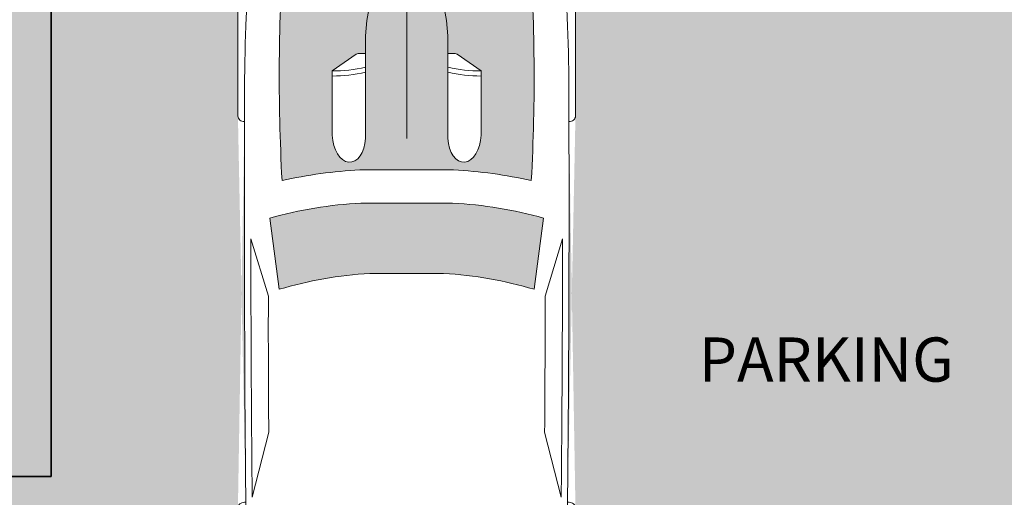
# Model space of a CAD drawing. Units: inches. Extents: x 2549 to 3108, y 1683 to 2362.
# Tile 5 of 30: x 2877 to 3018, y 1793 to 1861. Entities that reach past the tile are written whole.
import ezdxf

# ---------------------------------------------------------------- set-up
doc = ezdxf.new("R2010")
doc.units = ezdxf.units.IN
for name, color, linetype, lineweight in [('A-ANNO-DIMS', 2, 'Continuous', 18), ('A-AREA-IDEN', 7, 'Continuous', 18), ('A-FURN-PATT', 9, 'Continuous', 13), ('A-WALL', 7, 'Continuous', 35), ('A-WALL-PATT', 89, 'Continuous', 13), ('C-PKNG-VEHI', 8, 'Continuous', 18)]:
    doc.layers.add(name, color=color, linetype=linetype, lineweight=lineweight)
doc.layers.add('C-PKNG-VEHI-PATT', color=251, linetype='Continuous', lineweight=13, true_color=0x636466)
doc.layers.add('C-PVMT-PATT', color=9, linetype='Continuous', lineweight=13, true_color=0xc7c8ca)
doc.styles.get("Standard").update_dxf_attribs({"font": 'arial.ttf'})
doc.dimstyles.get("Standard").update_dxf_attribs({"dimtxt": 0.18, "dimasz": 0.18, "dimexe": 0.18, "dimexo": 0.0625, "dimgap": 0.09, "dimtad": 0, "dimtih": 1, "dimtoh": 1, "dimdec": 4, "dimzin": 0, "dimdsep": 46, "dimtxsty": 'Standard', "dimcen": 0.09, "dimadec": 0, "dimazin": 0, "dimtfac": 1, "dimtdec": 4, "dimtofl": 0, "dimtmove": 0, "dimatfit": 3, "dimfxl": 1, "dimtolj": 1, "dimtzin": 0, "dimarcsym": 0})

# ---------------------------------------------------------------- blocks, each defined once
blk = doc.blocks.new('*U11')
for p, q in [((46.55368679439944, 38.88847654282876), (22.35054758993934, 38.88847654282876)), ((136.6978032355602, 38.88847654282876), (160.90094244002, 38.88847654282867)), ((21.10406751471477, 37.40863046792069), (21.10406751471477, 36.83230215753705)), ((47.80016686962392, 37.39011648242055), (47.80016686962392, 37.40863046792069)), ((135.4513231603356, 37.07354110333037), (135.4513231603356, 37.40863046792069)), ((162.1474225152445, 37.40863046792049), (162.1474225152445, 36.77402019194128)), ((87.98532186932616, 31.87120872459877), (74.75900729854769, 35.92175679182955)), ((134.313356548143, 35.6043097713567), (119.2882629232503, 31.77757799177584)), ((186.4728846989705, -33.49860931502491), (186.4728846989718, 33.49860931502465)), ((188.3990091454065, -32.75868627757393), (188.3990091454077, 32.75868627757058)), ((70.0302824853563, 31.53613089391356), (86.40615155322342, 29.35124891408057)), ((138.4228833961707, 29.35124891408074), (157.2465674415997, 29.35124891408074)), ((186.4728846989718, 29.35124891408083), (167.0083537481071, 29.35124891408083)), ((164.515393597658, 26.39155676426461), (164.5153935976578, -26.39155676426503)), ((32.26591480791686, 11.62530558863241), (36.12873726252356, 17.16961494239206)), ((36.12873726252356, 17.16961494239206), (50.93891189819171, 17.16961494239206)), ((29.77279020470884, 9.505833383620029), (51.68362801571248, 9.505833383620029)), ((32.12291633764599, 9.505833383620029), (32.12291633764599, 11.15369945057711)), ((58.9167604809788, -10.77488335095668), (58.9167604809788, 10.77488335095617)), ((66.55009204259746, -10.5288681329018), (66.55009204259746, 10.52886813290129)), ((186.4728846989718, -10.5288681329018), (186.4728846989718, 10.52886813290129)), ((82.73706193978568, 8.496039918672748), (82.73706193978568, -8.49603991867258)), ((3.266462181856987, 6.128290093440767), (0.1022408397004821, 0.4060708604429806)), ((-4.43e-14, -2.558e-13), (51.68362801571248, -2.558e-13)), ((0.1022408397004821, -0.4060708604432933), (3.266462181856987, -6.128290093441194)), ((29.77279020470884, -9.50583338362054), (51.68362801571248, -9.50583338362054)), ((32.12291633764599, -9.50583338362054), (32.12291633764599, -11.15369945057762)), ((32.26591480791686, -11.62530558863292), (36.12873726252356, -17.16961494239257)), ((36.12873726252356, -17.16961494239257), (50.93891189819171, -17.16961494239257)), ((86.40615155322318, -29.35124891408145), (70.03028248535594, -31.53613089391442)), ((157.2465674415997, -29.35124891408117), (138.4228833961707, -29.35124891408126)), ((167.008353748107, -29.35124891408126), (186.4728846989707, -29.35124891408108)), ((87.98532186932607, -31.87120872459903), (74.7590072985476, -35.92175679182964)), ((134.3133565481428, -35.60430977135721), (119.2882629232503, -31.77757799177618)), ((21.10406751471477, -37.4086304679212), (21.10406751471477, -36.83230215753756)), ((47.80016686962392, -37.39011648242107), (47.80016686962392, -37.4086304679212)), ((135.4513231603355, -37.07354110333088), (135.4513231603355, -37.4086304679212)), ((162.1474225152445, -37.408630467921), (162.1474225152445, -36.77402019194179)), ((46.55368679439944, -38.88847654282927), (22.35054758993934, -38.88847654282927)), ((136.6978032355602, -38.88847654282927), (160.9009424400199, -38.88847654282918))]:
    blk.add_line(p, q)
for centre, major_axis, ratio, start_param, end_param in [((22.35054758993934, 37.40863046792072), (2.08e-14, -1.479846074908118), 0.842303869543976, 3.141592653589776, 4.712388980384677), ((46.55368679439944, 37.40863046792072), (2.2e-14, 1.479846074908118), 0.8423038695439758, -1.570796326794884, 1.73e-14), ((136.6978032355602, 37.40863046792072), (2.357e-13, -1.479846074908118), 0.842303869543976, 3.141592653589603, 4.712388980384554), ((160.90094244002, 37.40863046792052), (5.59e-14, 1.479846074908118), 0.842303869543976, -1.570796326794865, 4.44e-14), ((41.19115208863305, -490.8631038926156), (1.294e-13, 528.2339998381949), 0.8423038695439741, 0.0028100083536837, 0.0755983031096952), ((64.48199294511879, -10555.61767587835), (1.907644e-10, 10593.02630634627), 0.842303869543847, -0.0133969486112073, 0.0027970409639888), ((180.6280394947615, 35.8381667808375), (7.4e-14, 2.219769112362114), 0.8423038695439693, -0.0130174256259048, 1.249894140392862), ((64.48199294754608, -10556.35759891604), (1.349839377e-06, 10595.3130398087), 0.8423038681351469, -0.0133969484821159, -0.0130174254969711), ((183.9799245485226, 33.49860931502124), (3e-16, -2.959692149816168), 0.8423038695439952, 1.570796326796048, 3.128195704978389), ((183.9799245485216, 32.75868627756583), (8.56e-14, -5.246425615115243), 0.8423038695439737, 1.570796326795794, 3.128195704978164), ((266.0300214172791, -27.52442688366631), (1.966072e-10, 313.3077612809058), 0.8423038695435284, 1.367075990158062, 1.391760499156098), ((64.4819929449925, -10555.61767590795), (1.9177683e-09, -10591.54646030096), 0.8423038695482963, 3.133765086725325, 3.140440689641252), ((95.78879860270445, -3666.353346297651), (1.949864e-10, -3698.236159209632), 0.8423038695446962, 3.134048706297306, 3.14409775411291), ((37.47375371777758, -593.9621830607928), (6.21e-14, -623.32820996736), 0.8423038695439826, 3.09604606856106, 3.200911180495224), ((135.2911776514449, 5.387441675478555), (2.2715e-12, 81.77258453065997), 0.8423038695439563, 1.245306111696802, 1.507880129813836), ((259.1750197310735, -27.52442688366614), (1.506617e-10, -305.3028914627677), 0.8423038695443789, 4.528606069860317, 4.561837674556238), ((134.4003789125686, 5.387441675477674), (4.276e-13, -89.7774543484738), 0.84230386954398, 4.44948196380473, 4.652344057257214), ((149.595361812917, 2.799442537139299), (8.561e-13, -79.57966406425402), 0.842303869543983, 4.372215489277867, 4.640744122441986), ((17.08207736189386, -1.421e-13), (6.87e-14, 147.0179238898305), 0.8423038695439764, 4.511394369635731, 4.913383591133647), ((35.90576140732288, -1.421e-13), (6.87e-14, 147.0179238898305), 0.8423038695439764, 4.511394369635731, 4.913383591133647), ((167.0083537481071, 26.39155676426464), (1.394e-13, 2.959692149816236), 0.842303869543976, 5.55e-14, 1.57079632679492), ((-204.4946649195746, 52.39684969293512), (4.12053e-11, -250.9602162198571), 0.8423038695441164, 1.385369446298923, 1.434372047871027), ((13.03653510440275, 17.00972444508943), (1.2303e-12, 27.41599049210566), 0.8423038695439277, 4.435146050259648, 4.718221029521873), ((14.20086229321332, 17.00972444508943), (1.2303e-12, 27.41599049210566), 0.8423038695439277, 4.435146050259648, 4.718221029521873), ((50.7902773840875, 13.33772416300607), (6.340077547122382, -0.356608581037027), 0.6038335755719145, -1.39555193967809, 1.581314658479915), ((32.74615637525823, 11.15369945057713), (1.313e-13, 0.7399230374541176), 0.8423038695439091, 0.8797135699495516, 1.570796326795045), ((29.77279020470884, -46.66302566589627), (5.12e-14, 56.16885904951626), 0.842303869543976, 7e-16, 0.5903187773915901), ((0.6232400376122422, -1.421e-13), (1e-16, -0.7399230374541245), 0.842303869543842, 4.131459131953847, 5.293318828815531), ((29.77279020470884, 46.66302566589578), (4.004e-13, 56.16885904951626), 0.8423038695439734, 2.55127387619821, 3.141592653589801), ((-204.4946649195746, -52.39684969293552), (4.02945e-11, 250.9602162198562), 0.8423038695441192, -1.43437204787103, -1.385369446298926), ((149.5953618129329, -2.799442537137565), (4.0897e-12, -79.57966406427697), 0.8423038695439419, -1.499151468852248, -1.230622835688196), ((32.74615637525823, -11.1536994505777), (1.3e-13, -0.7399230374541176), 0.8423038695439093, 4.712388980384541, 5.403471737230034), ((13.03653510440275, -17.00972444508983), (1.2568e-12, -27.41599049210552), 0.8423038695439318, 1.564964277657711, 1.848039256919935), ((14.20086229321332, -17.00972444508983), (1.2568e-12, -27.41599049210552), 0.8423038695439318, 1.564964277657711, 1.848039256919935), ((134.4003789125684, -5.387441675478584), (4.2949e-12, -89.77745434847827), 0.8423038695439354, -1.510751403667474, -1.307889310215002), ((135.2911776514465, -5.387441675480715), (3.2038e-12, -81.77258453066244), 0.8423038695439492, -1.50788012981387, -1.245306111696839), ((259.1750197310694, 27.52442688365929), (1.08535e-11, 305.3028914629043), 0.8423038695439974, 1.721347632622872, 1.754579237318777), ((167.008353748107, -26.39155676426503), (1.02e-14, -2.959692149816192), 0.8423038695439885, 4.712388980384686, 6.283185307179581), ((266.0300214172791, 27.52442688366566), (8.75241e-11, 313.3077612806533), 0.8423038695441819, 1.749832154434603, 1.774516663432659), ((37.47375371777847, 593.9621830607904), (1.1693e-12, -623.3282099673584), 0.8423038695439528, -0.0593185269054384, 0.0455465850287298), ((95.78879860271888, 3666.35334629765), (1.637818e-10, -3698.236159209629), 0.8423038695447546, -0.0025051005232382, 0.007543947292366), ((183.9799245485216, -33.4986093150211), (9.3e-15, 2.959692149816141), 0.8423038695439732, 3.154989602201626, 4.71238898038339), ((183.9799245485177, -32.7586862775633), (2.428e-13, -5.246425615118353), 0.8423038695439808, 0.0133969486110846, 1.570796326792831), ((41.19115208863322, 490.8631038926152), (1.37757e-11, -528.2339998381949), 0.8423038695440652, -0.0755983031097181, -0.0028100083537155), ((64.48199294503607, 10555.61767590793), (1.6049794e-09, -10591.54646030094), 0.8423038695397146, 0.0011519639481523, 0.0078275668641468), ((22.35054758993934, -37.40863046792117), (2.2e-14, 1.479846074908118), 0.8423038695439758, 1.570796326794908, 3.14159265358981), ((64.48199294495228, 10555.61767590795), (6.117947e-10, 10593.02630637587), 0.8423038695458146, 3.138795612625926, 3.154989602201039), ((46.55368679439944, -37.40863046792117), (2.08e-14, -1.479846074908118), 0.842303869543976, -1.69e-14, 1.570796326794884), ((136.6978032355602, -37.40863046792109), (1.56e-14, -1.479846074908162), 0.8423038695440105, -1.570796326794875, -1.27e-14), ((160.9009424400199, -37.408630467921), (1.969e-13, 1.479846074908162), 0.8423038695440109, 3.141592653589951, 4.712388980384771), ((180.6280394947581, -35.83816678083949), (2.274e-13, -2.219769112363032), 0.8423038695439803, -1.249894138785958, 0.0130174256254374), ((64.48199294197605, 10556.3575989598), (9.365289701e-07, 10595.31303985772), 0.8423038705260315, 3.154610079306566, 3.154989602290631)]:
    blk.add_ellipse(centre, major_axis=major_axis, ratio=ratio, start_param=start_param, end_param=end_param)
at = {"extrusion": (0, 0, -1)}
blk.add_ellipse((50.7902773840875, -13.33772416300655), major_axis=(6.340077547122382, 0.3566085810370246), ratio=0.6038335755719145, start_param=-1.39555193967809, end_param=1.581314658479915, dxfattribs=at)
blk = doc.blocks.new('*D46')
at = {"layer": 'A-ANNO-DIMS', "color": 0, "lineweight": -2, "transparency": 16777216}
for p, q in [((2812.642666, 2140.461244), (2812.642666, 1683.443744)), ((3034.642666, 2134.461244), (3034.642666, 1683.443744)), ((2812.822666, 1683.623744), (2923.35320488131, 1683.623744)), ((3034.462666, 1683.623744), (2923.932127118691, 1683.623744))]:
    blk.add_line(p, q, dxfattribs=at)
at = {"layer": 'A-ANNO-DIMS', "color": 0, "transparency": 16777216}
for points in [[(2812.822666, 1683.653744), (2812.822666, 1683.593744), (2812.642666, 1683.623744)], [(3034.462666, 1683.653744), (3034.462666, 1683.593744), (3034.642666, 1683.623744)]]:
    blk.add_solid(points, dxfattribs=at)
at = {"layer": 'Defpoints', "color": 0, "transparency": 16777216}
for p in [(2812.642666, 2140.523744), (3034.642666, 2134.523744), (3034.642666, 1683.623744)]:
    blk.add_point(p, dxfattribs=at)
at = {"layer": 'A-ANNO-DIMS', "color": 0, "transparency": 16777216, "insert": (2923.642666000001, 1683.623744), "char_height": 0.18, "attachment_point": 5}
blk.add_mtext('\\A1;222', dxfattribs=at)

msp = doc.modelspace()

# ---------------------------------------------------------------- hatches: boundary and pattern name
at = {"layer": 'A-FURN-PATT', "transparency": 33554567}
h = msp.add_hatch(color=256, dxfattribs=at)
h.dxf.hatch_style = 1
h.paths.add_polyline_path([(2708.714672869869, 2271.673744486262), (2675.281339536536, 2271.673744486262), (2675.281339536536, 2262.040411152929), (2708.714672869869, 2262.040411152929)])
h.paths.add_polyline_path([(2980.824596989089, 2271.673744486262), (2947.391263655756, 2271.673744486262), (2947.391263655756, 2262.040411152929), (2980.824596989089, 2262.040411152929)])
h.paths.add_polyline_path([(2748.849609196547, 2101.638310911291), (2798.147998217048, 2101.638310911291), (2798.147998217048, 2111.424826549233), (2748.849609196547, 2111.424826549233)], flags=9)
h.paths.add_polyline_path([(2685.208067619545, 2101.488974631509), (2719.325307162104, 2101.488974631509), (2719.325307162104, 2111.281945754699), (2685.208067619545, 2111.281945754699)], flags=9)
h.paths.add_polyline_path([(2814.685179139321, 1907.132804880864), (2847.838399551318, 1907.132804880864), (2847.838399551318, 1916.925776004054), (2814.685179139321, 1916.925776004054)], flags=9)
h.paths.add_polyline_path([(2814.390575309562, 1835.586397562281), (2848.017197973174, 1835.586397562281), (2848.017197973174, 1845.379368685471), (2814.390575309562, 1845.379368685471)], flags=9)
h.paths.add_polyline_path([(2800.524456569608, 1759.167447237475), (2853.743476964851, 1759.167447237475), (2853.743476964851, 1768.953962875417), (2800.524456569608, 1768.953962875417)], flags=9)
h.paths.add_polyline_path([(2972.461062245805, 1807.33049128039), (3015.394342810494, 1807.33049128039), (3015.394342810494, 1817.117006918332), (2972.461062245805, 1817.117006918332)], flags=9)
h.paths.add_polyline_path([(2902.332650472062, 1888.673085326325), (2937.913133337796, 1888.673085326325), (2937.913133337796, 1898.466056449515), (2902.332650472062, 1898.466056449515)], flags=9)
h.paths.add_polyline_path([(2712.17793111998, 1878.903902566108), (2754.125674269943, 1878.903902566108), (2754.125674269943, 1888.69041820405), (2712.17793111998, 1888.69041820405)], flags=9)
h.paths.add_polyline_path([(2614.005606808349, 2012.811964980989), (2650.025062671036, 2012.811964980989), (2650.025062671036, 2022.437093487698), (2614.005606808349, 2022.437093487698)], flags=9)
h.paths.add_polyline_path([(2713.312922761346, 2003.164487508756), (2747.423706818656, 2003.164487508756), (2747.423706818656, 2012.951003146698), (2713.312922761346, 2012.951003146698)], flags=9)
h.paths.add_polyline_path([(2950.137937233872, 2001.693439459313), (2982.299164745893, 2001.693439459313), (2982.299164745893, 2011.479955097255), (2950.137937233872, 2011.479955097255)], flags=9)
h.paths.add_polyline_path([(2940.863994744806, 2238.553674899427), (2997.506574150595, 2238.553674899427), (2997.506574150595, 2248.346646022617), (2940.863994744806, 2248.346646022617)], flags=9)
h.paths.add_polyline_path([(2821.545730132573, 2202.834824551463), (2855.662969675132, 2202.834824551463), (2855.662969675132, 2212.627795674654), (2821.545730132573, 2212.627795674654)], flags=9)
h.paths.add_polyline_path([(2661.802564922812, 2238.624912952816), (2718.445144328601, 2238.624912952816), (2718.445144328601, 2248.417884076006), (2661.802564922812, 2248.417884076006)], flags=9)
h = msp.add_hatch(color=256, dxfattribs=at)
h.dxf.hatch_style = 1
h.paths.add_polyline_path([(2906.506430286822, 1905.214773716388), (2905.258354845315, 1904.38272342205), (2907.061130483047, 1900.777172146586), (2908.309205924554, 1901.609222440924)])
h.paths.add_polyline_path([(2936.521961741216, 1914.804377056317), (2935.27388629971, 1915.636427350655), (2932.63906036764, 1912.585576271416), (2933.887135809147, 1911.753525977078)])
h.paths.add_polyline_path([(2950.250791597791, 1905.651823818601), (2949.002716156284, 1906.483874112939), (2947.199940518553, 1902.878322837475), (2948.448015960059, 1902.046272543137)])
h.paths.add_polyline_path([(2958.571288994167, 1918.132569913166), (2956.907188405492, 1919.241970305616), (2952.469592522951, 1908.980025320303, 1.387427444474919), (2954.965744234361, 1907.315927313246)])
h.paths.add_polyline_path([(2945.258484284762, 1927.007773052769), (2943.594383696085, 1928.11717344522), (2934.996538511474, 1920.62873112851, 1.38742744447752), (2937.492687330065, 1918.964628782227)])
h.paths.add_polyline_path([(2748.849609196547, 2101.638310911291), (2798.147998217048, 2101.638310911291), (2798.147998217048, 2111.424826549233), (2748.849609196547, 2111.424826549233)], flags=9)
h.paths.add_polyline_path([(2685.208067619545, 2101.488974631509), (2719.325307162104, 2101.488974631509), (2719.325307162104, 2111.281945754699), (2685.208067619545, 2111.281945754699)], flags=9)
h.paths.add_polyline_path([(2814.685179139321, 1907.132804880864), (2847.838399551318, 1907.132804880864), (2847.838399551318, 1916.925776004054), (2814.685179139321, 1916.925776004054)], flags=9)
h.paths.add_polyline_path([(2814.390575309562, 1835.586397562281), (2848.017197973174, 1835.586397562281), (2848.017197973174, 1845.379368685471), (2814.390575309562, 1845.379368685471)], flags=9)
h.paths.add_polyline_path([(2800.524456569608, 1759.167447237475), (2853.743476964851, 1759.167447237475), (2853.743476964851, 1768.953962875417), (2800.524456569608, 1768.953962875417)], flags=9)
h.paths.add_polyline_path([(2972.461062245805, 1807.33049128039), (3015.394342810494, 1807.33049128039), (3015.394342810494, 1817.117006918332), (2972.461062245805, 1817.117006918332)], flags=9)
h.paths.add_polyline_path([(2902.332650472062, 1888.673085326325), (2937.913133337796, 1888.673085326325), (2937.913133337796, 1898.466056449515), (2902.332650472062, 1898.466056449515)], flags=9)
h.paths.add_polyline_path([(2712.17793111998, 1878.903902566108), (2754.125674269943, 1878.903902566108), (2754.125674269943, 1888.69041820405), (2712.17793111998, 1888.69041820405)], flags=9)
h.paths.add_polyline_path([(2614.005606808349, 2012.811964980989), (2650.025062671036, 2012.811964980989), (2650.025062671036, 2022.437093487698), (2614.005606808349, 2022.437093487698)], flags=9)
h.paths.add_polyline_path([(2713.312922761346, 2003.164487508756), (2747.423706818656, 2003.164487508756), (2747.423706818656, 2012.951003146698), (2713.312922761346, 2012.951003146698)], flags=9)
h.paths.add_polyline_path([(2950.137937233872, 2001.693439459313), (2982.299164745893, 2001.693439459313), (2982.299164745893, 2011.479955097255), (2950.137937233872, 2011.479955097255)], flags=9)
h.paths.add_polyline_path([(2940.863994744806, 2238.553674899427), (2997.506574150595, 2238.553674899427), (2997.506574150595, 2248.346646022617), (2940.863994744806, 2248.346646022617)], flags=9)
h.paths.add_polyline_path([(2821.545730132573, 2202.834824551463), (2855.662969675132, 2202.834824551463), (2855.662969675132, 2212.627795674654), (2821.545730132573, 2212.627795674654)], flags=9)
h.paths.add_polyline_path([(2661.802564922812, 2238.624912952816), (2718.445144328601, 2238.624912952816), (2718.445144328601, 2248.417884076006), (2661.802564922812, 2248.417884076006)], flags=9)
at = {"layer": 'A-WALL-PATT'}
h = msp.add_hatch(color=256, dxfattribs=at)
h.dxf.hatch_style = 1
h.paths.add_polyline_path([(2638.642666391656, 2272.523744486262), (3034.642666391656, 2272.523744486262), (3034.642666391656, 1936.523744486262), (3043.642666391656, 1936.523744486262), (3043.642666391656, 2281.523744486262), (2629.642666391656, 2281.523744486262), (2629.642666391656, 2074.523744486262), (2812.642666391655, 2074.523744486262), (2812.642666391655, 2140.523744486262), (2785.717675498527, 2140.523744486262), (2785.717675498527, 2134.523744486262), (2806.642666391656, 2134.523744486262), (2806.642666391656, 2080.523744486262), (2638.642666391656, 2080.523744486262)])
h.paths.add_polyline_path([(2638.642666391656, 1972.523744486262), (2662.642666391656, 1972.523744486262), (2662.642666391656, 2041.055679691546), (2653.642666391655, 2041.055679691546), (2653.642666391656, 1978.523744486262), (2629.642666391656, 1978.523744486262), (2629.642666391656, 1795.523744486262), (2662.642666391656, 1795.523744486262), (2881.642666391656, 1795.523744486262), (2881.642666391656, 1936.523744486262), (2965.935139880862, 1936.523744486262), (2965.935139880862, 1974.543933838007), (2959.935139880861, 1974.543933838007), (2959.935139880861, 1945.523744486262), (2881.642666391656, 1945.523744486262), (2872.642666391655, 1945.523744486262), (2872.642666391655, 1804.523744486262), (2662.642666391656, 1804.523744486262), (2638.642666391656, 1804.523744486262)])
at = {"layer": 'C-PKNG-VEHI-PATT'}
h = msp.add_hatch(color=256, dxfattribs=at)
h.dxf.hatch_style = 1
edge = h.paths.add_edge_path()
edge.add_ellipse((2935.725796552836, 1791.96404850691), major_axis=(-50.6600031146233, 6.78e-13), ratio=0.8423038695439883, start_angle=248.1650462032912, end_angle=265.7225790369452)
edge.add_line((2938.911028887629, 1834.550737322417), (2925.865275339109, 1834.550737322417))
edge.add_ellipse((2929.050507673901, 1791.964048506909), major_axis=(50.66000311462998, 7.2698e-12), ratio=0.8423038695438956, start_angle=94.27742096304536, end_angle=111.8349537966996)
edge.add_line((2912.850791291541, 1832.394679033669), (2914.204376096751, 1822.249450253823))
edge.add_ellipse((2930.653832861207, 1783.102276333115), major_axis=(-49.30143828149606, 1.1087e-12), ratio=0.8423038695440098, start_angle=-85.12993040286318, end_angle=-67.20808512241217, ccw=False)
edge.add_line((2927.124659327709, 1824.522535937876), (2937.65164489903, 1824.522535937876))
edge.add_ellipse((2934.122471365533, 1783.102276333124), major_axis=(49.30143828148681, 7.803e-13), ratio=0.8423038695439693, start_angle=67.20808512240922, end_angle=85.12993040286312, ccw=False)
edge.add_line((2950.571928129987, 1822.249450253823), (2951.925512935197, 1832.394679033669))
edge = h.paths.add_edge_path()
edge.add_ellipse((2903.479330909537, 1857.335124490177), major_axis=(-34.79790434319148, 3.2087e-12), ratio=0.8423038695440206, start_angle=180.0000000000052, end_angle=209.4385695979841)
edge.add_ellipse((2961.296973317201, 1857.335124490177), major_axis=(34.79790434319149, 1.2616e-12), ratio=0.8423038695439669, start_angle=150.5614304020187, end_angle=179.9999999999979)
edge.add_line((2926.49906897401, 1857.335124490177), (2926.49906897401, 1843.76085484809))
edge.add_ellipse((2924.125124210826, 1844.314306179491), major_axis=(-0.2209272451118966, 3.927824345135514), ratio=0.6038335755719296, start_angle=89.00201427502537, end_angle=253.65740804569998, ccw=False)
edge.add_line((2921.751179447642, 1844.222223668088), (2921.751179447642, 1853.39746861696))
edge.add_line((2921.751179447642, 1853.39746861696), (2925.26903797625, 1855.848425453852))
edge.add_ellipse((2925.478177919096, 1855.493055533625), major_axis=(0.4583993962922678, 2.303e-12), ratio=0.8423038695418179, start_angle=89.9999999997122, end_angle=134.4802108822853, ccw=False)
edge.add_line((2925.478177919095, 1855.879167118917), (2926.49906897401, 1855.879167118917))
edge.add_line((2926.49906897401, 1855.879167118917), (2926.49906897401, 1857.335124490177))
edge.add_ellipse((2961.296973317201, 1857.335124490177), major_axis=(34.79790434319149, 1.2616e-12), ratio=0.8423038695439669, start_angle=150.5614304020187, end_angle=179.999999999998, ccw=False)
edge.add_line((2932.388152113369, 1873.650056952746), (2932.388152113369, 1875.780055063896))
edge.add_ellipse((2932.388152113369, 1875.393943478604), major_axis=(0.4583993962904624, 1e-16), ratio=0.8423038695446395, start_angle=89.99999999999999, end_angle=127.9331304598429)
edge.add_line((2932.136581844764, 1875.716714504374), (2928.591534983032, 1873.756406364807))
edge.add_ellipse((2899.927094610101, 2002.469218934773), major_axis=(155.4756451483881, 9.82606e-11), ratio=0.842303869543439, start_angle=-80.74343399283458, end_angle=-77.44506735589891, ccw=False)
edge.add_ellipse((2949.440169726089, 1715.215149574257), major_axis=(-189.1421864819335, 9.35831e-11), ratio=0.8423038695443681, start_angle=-79.79046100282835, end_angle=-77.55537270652765)
edge.add_ellipse((3300.361430890526, 1852.564199885104), major_axis=(-386.1662101011402, 3.282e-12), ratio=0.8423038695438535, start_angle=-2.863714607837213, end_angle=2.198540565955553)
edge.add_ellipse((2929.050507673902, 1792.515918881865), major_axis=(-55.61920468847034, 9.624e-12), ratio=0.842303869544118, start_angle=-85.91758930883981, end_angle=-72.28004677724027, ccw=False)
edge.add_line((2925.712863234435, 1839.27976237288), (2939.063440992303, 1839.27976237288))
edge.add_ellipse((2935.725796552836, 1792.515918881865), major_axis=(55.61920468846977, 1.19088e-11), ratio=0.8423038695441256, start_angle=72.28004677723749, end_angle=85.91758930883759, ccw=False)
edge.add_ellipse((2564.414873336211, 1852.564199885105), major_axis=(-386.166210101141, 7.3121e-12), ratio=0.8423038695442235, start_angle=177.8014594340458, end_angle=182.8637146078386)
edge.add_ellipse((2915.336134500645, 1715.215149574254), major_axis=(189.1421864814668, 5.425418e-10), ratio=0.8423038695464061, start_angle=77.5553727063904, end_angle=79.79046100269107)
edge.add_ellipse((2964.849209616638, 2002.469218934773), major_axis=(-155.4756451483861, 9.70869e-11), ratio=0.8423038695434499, start_angle=77.44506735589852, end_angle=80.74343399283418, ccw=False)
edge.add_line((2936.184769243706, 1873.756406364807), (2932.639722381973, 1875.716714504375))
edge.add_ellipse((2932.388152113369, 1875.393943478604), major_axis=(0.4583993962904624, 1e-16), ratio=0.8423038695446395, start_angle=52.06686954015704, end_angle=89.99999999999999)
edge.add_line((2932.388152113369, 1875.780055063896), (2932.388152113369, 1873.650056952746))
edge.add_ellipse((2903.479330909537, 1857.335124490177), major_axis=(-34.79790434319148, 3.2087e-12), ratio=0.8423038695440206, start_angle=180.0000000000053, end_angle=209.4385695979841, ccw=False)
edge.add_line((2938.277235252728, 1857.335124490177), (2938.277235252728, 1855.879167118917))
edge.add_line((2938.277235252728, 1855.879167118917), (2939.405880844674, 1855.879167118917))
edge.add_ellipse((2939.298126307642, 1855.493055533625), major_axis=(-0.4583993962922676, 2.3028e-12), ratio=0.8423038695418185, start_angle=225.5197891177147, end_angle=270.00000000028786, ccw=False)
edge.add_line((2939.590297193029, 1855.790576266728), (2943.025124779096, 1853.39746861696))
edge.add_line((2943.025124779096, 1853.39746861696), (2943.025124779096, 1844.222223668088))
edge.add_ellipse((2940.651180015912, 1844.314306179491), major_axis=(0.2209272451118966, 3.927824345135514), ratio=0.6038335755719296, start_angle=106.3425919543001, end_angle=270.9979857249746, ccw=False)
edge.add_line((2938.277235252728, 1843.76085484809), (2938.277235252728, 1857.335124490177))
edge = h.paths.add_edge_path()
edge.add_ellipse((2932.388152113369, 1865.19731394932), major_axis=(91.08099646002908, 7.134e-13), ratio=0.8423038695439837, start_angle=256.4018653097688, end_angle=283.5981346902299, ccw=False)
edge.add_line((2914.204376096751, 1790.023884530285), (2914.204376096751, 1778.36217788565))
edge.add_ellipse((2932.388152113369, 1853.535607304685), major_axis=(91.08099646002908, 7.134e-13), ratio=0.8423038695439837, start_angle=256.4018653097688, end_angle=283.5981346902299)
edge.add_line((2950.571928129987, 1778.36217788565), (2950.571928129987, 1790.023884530285))
edge = h.paths.add_edge_path()
edge.add_ellipse((2948.738330544823, 1772.31452600415), major_axis=(1.833597585163715, 1.1861e-12), ratio=0.8423038695440299, start_angle=-3.70558e-11, end_angle=89.99999999996297)
edge.add_line((2948.738330544824, 1773.85897234532), (2916.037973681915, 1773.858972345321))
edge.add_ellipse((2916.037973681915, 1772.314526004151), major_axis=(1.833597585163716, 6.788e-13), ratio=0.84230386954403, start_angle=89.9999999999788, end_angle=179.9999999999787)
edge.add_line((2914.204376096751, 1772.314526004151), (2914.204376096751, 1760.255799913309))
edge.add_line((2914.204376096751, 1760.255799913309), (2950.571928129987, 1760.255799913308))
edge.add_line((2950.571928129987, 1760.255799913308), (2950.571928129987, 1772.31452600415))
h.paths.add_polyline_path([(2748.849609196547, 2101.638310911291), (2798.147998217048, 2101.638310911291), (2798.147998217048, 2111.424826549233), (2748.849609196547, 2111.424826549233)], flags=9)
h.paths.add_polyline_path([(2685.208067619545, 2101.488974631509), (2719.325307162104, 2101.488974631509), (2719.325307162104, 2111.281945754699), (2685.208067619545, 2111.281945754699)], flags=9)
h.paths.add_polyline_path([(2814.685179139321, 1907.132804880864), (2847.838399551318, 1907.132804880864), (2847.838399551318, 1916.925776004054), (2814.685179139321, 1916.925776004054)], flags=9)
h.paths.add_polyline_path([(2814.390575309562, 1835.586397562281), (2848.017197973174, 1835.586397562281), (2848.017197973174, 1845.379368685471), (2814.390575309562, 1845.379368685471)], flags=9)
h.paths.add_polyline_path([(2800.524456569608, 1759.167447237475), (2853.743476964851, 1759.167447237475), (2853.743476964851, 1768.953962875417), (2800.524456569608, 1768.953962875417)], flags=9)
h.paths.add_polyline_path([(2972.461062245805, 1807.33049128039), (3015.394342810494, 1807.33049128039), (3015.394342810494, 1817.117006918332), (2972.461062245805, 1817.117006918332)], flags=9)
h.paths.add_polyline_path([(2902.332650472062, 1888.673085326325), (2937.913133337796, 1888.673085326325), (2937.913133337796, 1898.466056449515), (2902.332650472062, 1898.466056449515)], flags=9)
h.paths.add_polyline_path([(2712.17793111998, 1878.903902566108), (2754.125674269943, 1878.903902566108), (2754.125674269943, 1888.69041820405), (2712.17793111998, 1888.69041820405)], flags=9)
h.paths.add_polyline_path([(2614.005606808349, 2012.811964980989), (2650.025062671036, 2012.811964980989), (2650.025062671036, 2022.437093487698), (2614.005606808349, 2022.437093487698)], flags=9)
h.paths.add_polyline_path([(2713.312922761346, 2003.164487508756), (2747.423706818656, 2003.164487508756), (2747.423706818656, 2012.951003146698), (2713.312922761346, 2012.951003146698)], flags=9)
h.paths.add_polyline_path([(2950.137937233872, 2001.693439459313), (2982.299164745893, 2001.693439459313), (2982.299164745893, 2011.479955097255), (2950.137937233872, 2011.479955097255)], flags=9)
h.paths.add_polyline_path([(2940.863994744806, 2238.553674899427), (2997.506574150595, 2238.553674899427), (2997.506574150595, 2248.346646022617), (2940.863994744806, 2248.346646022617)], flags=9)
h.paths.add_polyline_path([(2821.545730132573, 2202.834824551463), (2855.662969675132, 2202.834824551463), (2855.662969675132, 2212.627795674654), (2821.545730132573, 2212.627795674654)], flags=9)
h.paths.add_polyline_path([(2661.802564922812, 2238.624912952816), (2718.445144328601, 2238.624912952816), (2718.445144328601, 2248.417884076006), (2661.802564922812, 2248.417884076006)], flags=9)
at = {"layer": 'C-PVMT-PATT'}
h = msp.add_hatch(color=256, dxfattribs=at)
h.dxf.hatch_style = 1
h.paths.add_polyline_path([(3067.642666391656, 2305.523744486262), (2605.642666391656, 2305.523744486262), (2605.642666391656, 2074.523744486262), (2629.642666391656, 2074.523744486262), (2629.642666391656, 2281.523744486262), (3043.642666391656, 2281.523744486262), (3043.642666391656, 1885.523744486263), (3043.642666391656, 1872.874514030248), (3031.167181590035, 1872.874514030248), (3031.167181590035, 1862.573058982011), (2995.805391311171, 1862.573058982011), (2995.805391311171, 1872.874514030248), (2983.175155144805, 1872.874514030248), (2983.175155144805, 1885.523744486262), (2881.642666391656, 1885.523744486263), (2881.642666391656, 1795.523744486262), (2751.09773888662, 1795.523744486262), (2751.09773888662, 1761.523744486262), (2786.157685455576, 1761.523744486262), (2786.157685455577, 1723.523744486262), (2881.839988255281, 1723.523744486262), (2881.839988255281, 1714.523744486262), (3067.642666391656, 1714.523744486262), (3067.642666391656, 1723.523744486262)])
edge = h.paths.add_edge_path(flags=16)
edge.add_ellipse((2949.440169726093, 1710.96831784248), major_axis=(-194.1013880556022, 3.100242e-10), ratio=0.8423038695451509, start_angle=-77.87403444762441, end_angle=-76.21947101041059, ccw=False)
edge.add_ellipse((2949.440169726089, 1715.215149574257), major_axis=(-189.1421864819335, 9.35831e-11), ratio=0.8423038695443681, start_angle=-79.7904610028283, end_angle=-77.55537270652758, ccw=False)
edge.add_ellipse((2899.927094610101, 2002.469218934773), major_axis=(155.4756451483881, 9.82606e-11), ratio=0.842303869543439, start_angle=-80.74343399283462, end_angle=-77.44506735589897)
edge.add_line((2928.591534983032, 1873.756406364807), (2932.388152113369, 1875.855825569603))
edge.add_line((2932.388152113369, 1875.855825569603), (2936.184769243706, 1873.756406364807))
edge.add_ellipse((2964.849209616638, 2002.469218934773), major_axis=(-155.4756451483861, 9.70869e-11), ratio=0.8423038695434499, start_angle=77.4450673558985, end_angle=80.74343399283416)
edge.add_ellipse((2915.336134500645, 1715.215149574254), major_axis=(189.1421864814668, 5.425418e-10), ratio=0.8423038695464061, start_angle=77.55537270639041, end_angle=79.79046100269102, ccw=False)
edge.add_ellipse((2915.336134500645, 1710.96831784248), major_axis=(-194.1013880561466, 2.794238e-10), ratio=0.8423038695428703, start_angle=256.2194710105847, end_angle=257.8740344477983, ccw=False)
edge.add_ellipse((2628.287132012546, 1850.261185811051), major_axis=(-327.2531525161749, 1.24457e-11), ratio=0.8423038695440036, start_angle=182.1799503136474, end_angle=183.6504275857012, ccw=False)
edge.add_ellipse((2955.563661936079, 1861.933375066942), major_axis=(-0.9167987925820851, 6.203e-13), ratio=0.8423038695438211, start_angle=180.0000000000388, end_angle=270.00000000003877, ccw=False)
edge.add_line((2956.480460728661, 1862.385732927092), (2956.480460728661, 1846.486613953928))
edge.add_ellipse((2955.563661936079, 1846.938971814078), major_axis=(-0.9167987925816303, 6.983e-13), ratio=0.8423038695442389, start_angle=90.0000000000436, end_angle=180.0000000000437, ccw=False)
edge.add_ellipse((-3607.060581297885, 1835.831972437108), major_axis=(-6562.624243233964, 2.000376e-10), ratio=0.8423038695434055, start_angle=179.6161332212093, end_angle=180.0902290885961, ccw=False)
edge.add_ellipse((2955.563661936079, 1791.092611498023), major_axis=(0.9167987925816303, 1.8053e-12), ratio=0.8423038695442389, start_angle=-1.127773430198431e-10, end_angle=89.99999999988711, ccw=False)
edge.add_line((2956.480460728661, 1791.544969358173), (2956.480460728661, 1775.645850385008))
edge.add_ellipse((2955.563661936079, 1776.098208245159), major_axis=(0.9167987925816303, 5.91e-14), ratio=0.8423038695442391, start_angle=269.9999999999963, end_angle=359.9999999999963, ccw=False)
edge.add_ellipse((-3607.060581297885, 1835.831972437108), major_axis=(-6562.624243233964, 2.000376e-10), ratio=0.8423038695434055, start_angle=179.3813568036826, end_angle=179.4717285281838, ccw=False)
edge.add_ellipse((2954.590723441648, 1763.876816393945), major_axis=(-1.375198188872997, 3.586e-13), ratio=0.8423038695436877, start_angle=179.3717627838213, end_angle=248.4647566010281, ccw=False)
edge.add_ellipse((-3607.518980694323, 1835.831972435604), major_axis=(-6564.040927375597, 4.0829067806e-06), ratio=0.8423038626957529, start_angle=179.3534459385899, end_angle=179.371762819423, ccw=False)
edge.add_ellipse((2952.682914207262, 1761.800246254478), major_axis=(3.250281735962, 3.921e-13), ratio=0.8423038695438826, start_angle=-89.99999999994031, end_angle=-0.6465540970884831, ccw=False)
edge.add_line((2952.682914207266, 1759.06252137117), (2912.093390019471, 1759.062521371171))
edge.add_ellipse((2912.093390019478, 1761.800246254481), major_axis=(3.250281735963338, 1.2841e-12), ratio=0.8423038695440954, start_angle=180.6465540970387, end_angle=269.99999999984414, ccw=False)
edge.add_ellipse((9472.295284948175, 1835.831972439052), major_axis=(-6564.040927413921, 8.323842912e-07), ratio=0.8423038709559154, start_angle=0.6282372235086768, end_angle=0.646554104341817, ccw=False)
edge.add_ellipse((2910.185580785089, 1763.876816393947), major_axis=(1.375198188873441, 9.687e-13), ratio=0.8423038695438604, start_angle=111.53524350397811, end_angle=180.6282372161342, ccw=False)
edge.add_ellipse((9471.836885542962, 1835.831972437208), major_axis=(-6562.624243252301, 3.836442e-10), ratio=0.8423038695462286, start_angle=0.5282714718206876, end_angle=0.6465540970643247, ccw=False)
edge.add_ellipse((2909.212642290659, 1776.098208245159), major_axis=(-0.9167987925820851, 6.203e-13), ratio=0.8423038695438211, start_angle=3.8824055081931874e-11, end_angle=90.00000000003882, ccw=False)
edge.add_line((2908.295843498077, 1775.645850385009), (2908.295843498077, 1791.544969358173))
edge.add_ellipse((2909.212642290659, 1791.092611498023), major_axis=(-0.9167987925820851, 4.868e-13), ratio=0.8423038695438213, start_angle=-89.99999999996948, end_angle=3.041122909053229e-11, ccw=False)
edge.add_ellipse((9471.836885542962, 1835.831972437208), major_axis=(-6562.624243252301, 3.836442e-10), ratio=0.8423038695462286, start_angle=-0.09022908858980827, end_angle=0.38386677879560693, ccw=False)
edge.add_ellipse((2909.212642290658, 1846.938971814078), major_axis=(-0.9167987925816306, 1.1661e-12), ratio=0.8423038695442389, start_angle=7.287326297955588e-11, end_angle=90.00000000007287, ccw=False)
edge.add_line((2908.295843498077, 1846.486613953928), (2908.295843498077, 1862.385732927092))
edge.add_ellipse((2909.212642290658, 1861.933375066942), major_axis=(0.9167987925816303, 1.1659e-12), ratio=0.8423038695442391, start_angle=89.99999999992713, end_angle=179.9999999999272, ccw=False)
edge.add_ellipse((3236.489172214191, 1850.261185811051), major_axis=(327.2531525161745, 3.33005e-11), ratio=0.8423038695444386, start_angle=176.3495724142951, end_angle=177.820049686349, ccw=False)
edge = h.paths.add_edge_path(flags=0)
edge.add_ellipse((2903.479330909537, 1857.335124490177), major_axis=(-34.79790434319148, 3.2087e-12), ratio=0.8423038695440206, start_angle=180.0000000000053, end_angle=209.4385695979841, ccw=False)
edge.add_line((2938.277235252728, 1857.335124490177), (2938.277235252728, 1855.879167118917))
edge.add_line((2938.277235252728, 1855.879167118917), (2939.463142736354, 1855.879167118917))
edge.add_line((2939.463142736354, 1855.879167118917), (2943.025124779096, 1853.39746861696))
edge.add_line((2943.025124779096, 1853.39746861696), (2943.025124779096, 1844.222223668088))
edge.add_ellipse((2940.651180015912, 1844.314306179491), major_axis=(0.2209272451118966, 3.927824345135514), ratio=0.6038335755719296, start_angle=106.3425919543001, end_angle=270.9979857249746, ccw=False)
edge.add_line((2938.277235252728, 1843.76085484809), (2938.277235252728, 1857.335124490177))
edge.add_ellipse((2903.479330909537, 1857.335124490177), major_axis=(-34.79790434319148, 3.2087e-12), ratio=0.8423038695440206, start_angle=180.0000000000052, end_angle=209.4385695979841)
edge.add_ellipse((2961.296973317201, 1857.335124490177), major_axis=(34.79790434319149, 1.2616e-12), ratio=0.8423038695439669, start_angle=150.5614304020187, end_angle=179.9999999999979)
edge.add_line((2926.49906897401, 1857.335124490177), (2926.49906897401, 1843.76085484809))
edge.add_ellipse((2924.125124210826, 1844.314306179491), major_axis=(-0.2209272451118966, 3.927824345135514), ratio=0.6038335755719296, start_angle=89.00201427502537, end_angle=253.65740804569998, ccw=False)
edge.add_line((2921.751179447642, 1844.222223668088), (2921.751179447642, 1853.39746861696))
edge.add_line((2921.751179447642, 1853.39746861696), (2925.313161490385, 1855.879167118917))
edge.add_line((2925.313161490385, 1855.879167118917), (2926.49906897401, 1855.879167118917))
edge.add_line((2926.49906897401, 1855.879167118917), (2926.49906897401, 1857.335124490177))
edge.add_ellipse((2961.296973317201, 1857.335124490177), major_axis=(34.79790434319149, 1.2616e-12), ratio=0.8423038695439669, start_angle=150.5614304020187, end_angle=179.999999999998, ccw=False)
edge = h.paths.add_edge_path(flags=0)
edge.add_ellipse((2929.050507673901, 1791.964048506909), major_axis=(50.66000311462998, 7.2698e-12), ratio=0.8423038695438956, start_angle=94.2774209630453, end_angle=111.8349537966997, ccw=False)
edge.add_line((2925.865275339109, 1834.550737322417), (2938.911028887629, 1834.550737322417))
edge.add_ellipse((2935.725796552836, 1791.96404850691), major_axis=(-50.6600031146233, 6.78e-13), ratio=0.8423038695439883, start_angle=248.16504620329118, end_angle=265.72257903694526, ccw=False)
edge.add_line((2951.925512935197, 1832.394679033669), (2950.571928129987, 1822.249450253823))
edge.add_ellipse((2934.122471365533, 1783.102276333124), major_axis=(49.30143828148681, 7.803e-13), ratio=0.8423038695439693, start_angle=67.20808512240917, end_angle=85.12993040286312)
edge.add_line((2937.651644899029, 1824.522535937876), (2927.12465932771, 1824.522535937876))
edge.add_ellipse((2930.653832861207, 1783.102276333115), major_axis=(-49.30143828149606, 1.1087e-12), ratio=0.8423038695440098, start_angle=-85.12993040286322, end_angle=-67.20808512241221)
edge.add_line((2914.204376096751, 1822.249450253823), (2912.850791291541, 1832.394679033669))
edge = h.paths.add_edge_path(flags=0)
edge.add_line((2910.133794844343, 1829.46512489105), (2912.643202843121, 1821.271117801794))
edge.add_ellipse((5203.77865552976, 1816.436683891122), major_axis=(-2291.142641748503, 9.8835e-11), ratio=0.8423038695495838, start_angle=-0.1208973690305054, end_angle=0.3640763488925343)
edge.add_line((2912.701209242743, 1801.878223466977), (2910.33046059899, 1792.569831244782))
edge.add_ellipse((9471.836885542954, 1835.831972437156), major_axis=(-6561.70744445971, 7.61654e-11), ratio=0.8423038695443023, start_angle=0.055594313499796044, end_angle=0.37776419391019544, ccw=False)
edge = h.paths.add_edge_path(flags=0)
edge.add_ellipse((-3607.060581316224, 1835.831972437187), major_axis=(6561.707444459722, 1.43187e-10), ratio=0.8423038695443235, start_angle=-0.37776419391110494, end_angle=-0.05559431350059185, ccw=False)
edge.add_line((2954.445843627751, 1792.569831244769), (2952.075094983995, 1801.878223466976))
edge.add_ellipse((660.9976486969767, 1816.436683891133), major_axis=(2291.142641748505, 5.276994e-10), ratio=0.842303869552366, start_angle=-0.3640763489035208, end_angle=0.1208973690194708)
edge.add_line((2952.133101383619, 1821.2711178018), (2954.642509382395, 1829.46512489105))
edge = h.paths.add_edge_path(flags=0)
edge.add_ellipse((2932.388152113369, 1865.19731394932), major_axis=(91.08099646002908, 7.134e-13), ratio=0.8423038695439837, start_angle=256.4018653097688, end_angle=283.5981346902299)
edge.add_line((2950.571928129987, 1790.023884530285), (2950.571928129987, 1778.362177885651))
edge.add_ellipse((2932.388152113369, 1853.535607304685), major_axis=(91.08099646002908, 7.134e-13), ratio=0.8423038695439837, start_angle=256.4018653097688, end_angle=283.5981346902299, ccw=False)
edge.add_line((2914.204376096751, 1778.362177885651), (2914.204376096751, 1790.023884530285))
edge = h.paths.add_edge_path(flags=0)
edge.add_line((2916.037973681915, 1773.858972345321), (2948.738330544823, 1773.85897234532))
edge.add_ellipse((2948.738330544823, 1772.31452600415), major_axis=(1.833597585163715, 1.1861e-12), ratio=0.8423038695440299, start_angle=-3.7118752516107634e-11, end_angle=89.999999999963, ccw=False)
edge.add_line((2950.571928129987, 1772.31452600415), (2950.571928129987, 1760.255799913308))
edge.add_line((2950.571928129987, 1760.255799913308), (2914.204376096751, 1760.255799913309))
edge.add_line((2914.204376096751, 1760.255799913309), (2914.204376096751, 1772.314526004151))
edge.add_ellipse((2916.037973681915, 1772.314526004151), major_axis=(1.833597585163716, 6.788e-13), ratio=0.84230386954403, start_angle=89.9999999999788, end_angle=179.9999999999788, ccw=False)
h.paths.add_polyline_path([(2629.642666391656, 1978.523744486262), (2605.642666391656, 1978.523744486262), (2605.642666391656, 1723.523744486262), (2629.642666391656, 1723.523744486262), (2629.642666391656, 1795.523744486262)], flags=17)
h.paths.add_polyline_path([(2800.524456569608, 1759.167447237475), (2853.743476964851, 1759.167447237475), (2853.743476964851, 1768.953962875417), (2800.524456569608, 1768.953962875417)], flags=24)
h.paths.add_polyline_path([(2972.461062245805, 1807.33049128039), (3015.394342810494, 1807.33049128039), (3015.394342810494, 1817.117006918332), (2972.461062245805, 1817.117006918332)], flags=24)

# ---------------------------------------------------------------- linework, layer by layer
at = {"layer": 'A-WALL'}
msp.add_line((2881.642666391656, 1795.523744486262), (2881.642666391656, 1936.523744486262), dxfattribs=at)
msp.add_lwpolyline([(2629.642666391656, 1795.523744486262), (2662.642666391656, 1795.523744486262), (2881.642666391656, 1795.523744486262)], dxfattribs=at)

# ---------------------------------------------------------------- block references
at = {"layer": 'C-PKNG-VEHI', "xscale": 0.6195230761677903, "yscale": 0.6195230761677903, "zscale": 0.6195230761677903, "rotation": 270}
msp.add_blockref('*U11', (2932.388152113369, 1875.780055063896), dxfattribs=at)

# ---------------------------------------------------------------- texts
at = {"layer": 'A-AREA-IDEN'}
msp.add_text('PARKING', height=6.309160916984183, dxfattribs=at).set_placement((2974.092148185462, 1809.069168640869))

# ---------------------------------------------------------------- dimensions: what is measured, and where the dimension line sits
at = {"layer": 'A-ANNO-DIMS'}
dim = msp.add_linear_dim(base=(3034.642666, 1683.623744), p1=(2812.642666, 2140.523744), p2=(3034.642666, 2134.523744), dimstyle='Standard', override={"dimdec": 0, "dimlfac": 1, "dimrnd": 0, "dimzin": 0, "dimdsep": 46, "dimlunit": 2}, dxfattribs=at)
dim.commit()
dim.dimension.update_dxf_attribs({"geometry": '*D46', "text_midpoint": (2923.642666000001, 1683.623744)})

doc.saveas('drawing.dxf')
